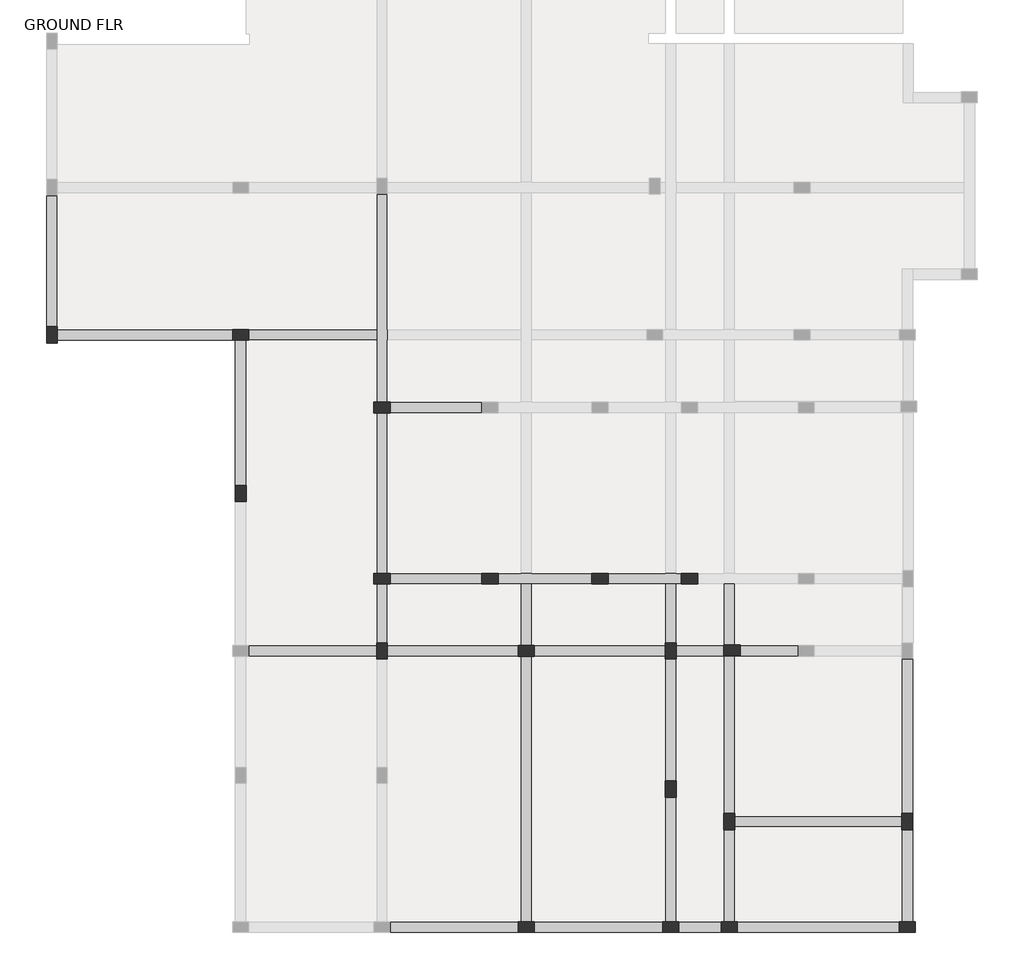
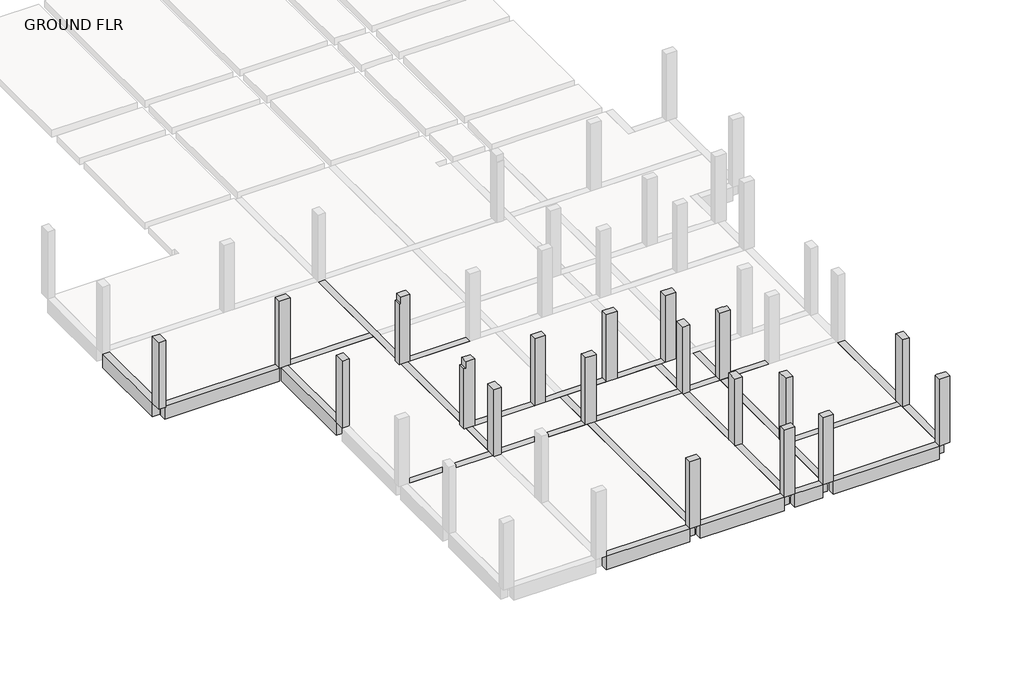
# One storey, part 2 of 5: 30 beams, 19 columns.
"""IFC4 building model written with IfcOpenShell, lengths in millimetres."""

from ifc_helpers import new_model, si_unit, frame, origin, place, context, project, spatial, polyline, outline, extrude, faceted_brep, element, save

model = new_model("IFC4")

# Units and contexts
model_context = context("Model", 3, world=origin())
ifc_project = project(units=[si_unit("LENGTHUNIT", "METRE", prefix="MILLI")], contexts=[model_context])

# Site, building, storey
site = spatial("IfcSite", under=ifc_project)
building = spatial("IfcBuilding", under=site)
storey = spatial("IfcBuildingStorey", under=building, Name="GROUND FLR", Elevation=0.0)

# Beams
placement = place(None, origin())
element("IfcBeam", 1, ObjectType="M_Concrete-Rectangular Beam : 300 x 600mm", at=placement, inside=storey, context=model_context, shape_type="SweptSolid", body=[
    extrude(outline(polyline([(-10828.8105653, -2764.4535766), (-11128.8105653, -2764.4535766), (-11128.8105653, 876.1713929), (-10828.8105653, 876.1713929), (-10828.8105653, -2764.4535766)])), frame((0.0, 0.0, -600.0), z_axis=(0.0, 0.0, 1.0), x_axis=(1.0, 0.0, 0.0)), (0.0, 0.0, 1.0), 600.0),
])
element("IfcBeam", 2, ObjectType="M_Concrete-Rectangular Beam : 300 x 600mm", at=placement, inside=storey, context=model_context, shape_type="Brep", body=[
    faceted_brep([(-5963.8105653, -3139.4535766, 0.0), (-5963.8105653, -2839.4535766, 0.0), (-10828.8105653, -2839.4535766, 0.0), (-10828.8105653, -3139.4535766, 0.0), (-5963.8105653, -3139.4535766, -600.0), (-10828.8105653, -3139.4535766, -600.0), (-5963.8105653, -2839.4535766, -600.0), (-10828.8105653, -2839.4535766, -600.0), (-5963.8105653, -2839.4535766, -300.0), (-10828.8105653, -2839.4535766, -300.0)], [[[0, 1, 2, 3]], [[4, 0, 3, 5]], [[6, 4, 5, 7]], [[2, 1, 8, 6, 7, 9]], [[1, 0, 4, 6, 8]], [[3, 2, 9, 7, 5]]]),
])
element("IfcBeam", 3, ObjectType="M_Concrete-Rectangular Beam : 300 x 600mm", at=placement, inside=storey, context=model_context, shape_type="Brep", body=[
    faceted_brep([(-5588.8105653, -7169.0760584, 0.0), (-5588.8105653, -3139.4535766, 0.0), (-5888.8105653, -3139.4535766, 0.0), (-5888.8105653, -7169.0760584, 0.0), (-5888.8105653, -3139.4535766, -600.0), (-5888.8105653, -7169.0760584, -600.0), (-5588.8105653, -3139.4535766, -600.0), (-5588.8105653, -7169.0760584, -600.0), (-5588.8105653, -7169.0760584, -300.0), (-5588.8105653, -3139.4535766, -300.0)], [[[0, 1, 2, 3]], [[3, 2, 4, 5]], [[5, 4, 6, 7]], [[1, 0, 8, 7, 6, 9]], [[6, 4, 2, 1, 9]], [[0, 3, 5, 7, 8]]]),
])
element("IfcBeam", 4, ObjectType="M_Concrete-Rectangular Beam : 300 x 600mm", at=placement, inside=storey, context=model_context, shape_type="SweptSolid", body=[
    extrude(outline(polyline([(1949.7296816, -19272.5304373), (1949.7296816, -19572.5304373), (-1596.7865686, -19572.5304373), (-1596.7865686, -19272.5304373), (1949.7296816, -19272.5304373)])), frame((0.0, 0.0, -600.0), z_axis=(0.0, 0.0, 1.0), x_axis=(1.0, 0.0, 0.0)), (0.0, 0.0, 1.0), 600.0),
])
element("IfcBeam", 5, ObjectType="M_Concrete-Rectangular Beam : 300 x 600mm", at=placement, inside=storey, context=model_context, shape_type="SweptSolid", body=[
    extrude(outline(polyline([(5957.5248054, -19272.5304373), (5957.5248054, -19572.5304373), (2399.7296816, -19572.5304373), (2399.7296816, -19272.5304373), (5957.5248054, -19272.5304373)])), frame((0.0, 0.0, -600.0), z_axis=(0.0, 0.0, 1.0), x_axis=(1.0, 0.0, 0.0)), (0.0, 0.0, 1.0), 600.0),
])
element("IfcBeam", 6, ObjectType="M_Concrete-Rectangular Beam : 300 x 600mm", at=placement, inside=storey, context=model_context, shape_type="SweptSolid", body=[
    extrude(outline(polyline([(7581.8679014, -19272.5304373), (7581.8679014, -19572.5304373), (6407.5248054, -19572.5304373), (6407.5248054, -19272.5304373), (7581.8679014, -19272.5304373)])), frame((0.0, 0.0, -600.0), z_axis=(0.0, 0.0, 1.0), x_axis=(1.0, 0.0, 0.0)), (0.0, 0.0, 1.0), 600.0),
])
element("IfcBeam", 7, ObjectType="M_Concrete-Rectangular Beam : 300 x 600mm", at=placement, inside=storey, context=model_context, shape_type="SweptSolid", body=[
    extrude(outline(polyline([(12524.1163908, -19272.5304373), (12524.1163908, -19572.5304373), (8031.8679014, -19572.5304373), (8031.8679014, -19272.5304373), (12524.1163908, -19272.5304373)])), frame((0.0, 0.0, -600.0), z_axis=(0.0, 0.0, 1.0), x_axis=(1.0, 0.0, 0.0)), (0.0, 0.0, 1.0), 600.0),
])
element("IfcBeam", 8, ObjectType="M_Concrete-Rectangular Beam : 300 x 600mm", at=placement, inside=storey, context=model_context, shape_type="Brep", body=[
    faceted_brep([(12599.1163908, -19272.5304373, 0.0), (12899.1163908, -19272.5304373, 0.0), (12899.1163908, -16719.1579597, 0.0), (12599.1163908, -16719.1579597, 0.0), (12899.1163908, -19272.5304373, -600.0), (12899.1163908, -16719.1579597, -600.0), (12599.1163908, -19272.5304373, -600.0), (12599.1163908, -16719.1579597, -600.0), (12599.1163908, -16719.1579597, -300.0), (12599.1163908, -19272.5304373, -300.0)], [[[0, 1, 2, 3]], [[1, 4, 5, 2]], [[4, 6, 7, 5]], [[0, 3, 8, 7, 6, 9]], [[6, 4, 1, 0, 9]], [[3, 2, 5, 7, 8]]]),
])
element("IfcBeam", 9, ObjectType="M_Concrete-Rectangular Beam : 300 x 600mm", at=placement, inside=storey, context=model_context, shape_type="Brep", body=[
    faceted_brep([(12599.1163908, -16269.1579597, 0.0), (12899.1163908, -16269.1579597, 0.0), (12899.1163908, -11982.8970059, 0.0), (12599.1163908, -11982.8970059, 0.0), (12899.1163908, -16269.1579597, -600.0), (12899.1163908, -11982.8970059, -600.0), (12599.1163908, -16269.1579597, -600.0), (12599.1163908, -11982.8970059, -600.0), (12599.1163908, -11982.8970059, -300.0), (12599.1163908, -16269.1579597, -300.0)], [[[0, 1, 2, 3]], [[1, 4, 5, 2]], [[4, 6, 7, 5]], [[0, 3, 8, 7, 6, 9]], [[6, 4, 1, 0, 9]], [[3, 2, 5, 7, 8]]]),
])
element("IfcBeam", 10, ObjectType="M_Concrete-Rectangular Beam : 300 x 600mm", at=placement, inside=storey, context=model_context, shape_type="Brep", body=[
    faceted_brep([(-1971.7865686, -9907.1078267, 0.0), (-1971.7865686, -11532.8970059, 0.0), (-1671.7865686, -11532.8970059, 0.0), (-1671.7865686, -9907.1078267, 0.0), (-1671.7865686, -11532.8970059, -300.0), (-1671.7865686, -11532.8970059, -600.0), (-1671.7865686, -9907.1078267, -600.0), (-1671.7865686, -9907.1078267, -300.0), (-1971.7865686, -11532.8970059, -600.0), (-1971.7865686, -9907.1078267, -600.0), (-1971.7865686, -9907.1078267, -300.0), (-1971.7865686, -11532.8970059, -300.0)], [[[0, 1, 2, 3]], [[3, 2, 4, 5, 6, 7]], [[6, 5, 8, 9]], [[1, 0, 10, 9, 8, 11]], [[0, 3, 7, 6, 9, 10]], [[8, 5, 4, 2, 1, 11]]]),
])
element("IfcBeam", 11, ObjectType="M_Concrete-Rectangular Beam : 300 x 600mm", at=placement, inside=storey, context=model_context, shape_type="Brep", body=[
    faceted_brep([(-1671.7865686, 916.1713929, 0.0), (-1971.7865686, 916.1713929, 0.0), (-1971.7865686, -2839.4535766, 0.0), (-1971.7865686, -3139.4535766, 0.0), (-1971.7865686, -4851.6229916, 0.0), (-1671.7865686, -4851.6229916, 0.0), (-1671.7865686, -3139.4535766, 0.0), (-1671.7865686, -2839.4535766, 0.0), (-1971.7865686, 916.1713929, -600.0), (-1971.7865686, -2839.4535766, -600.0), (-1971.7865686, -3139.4535766, -600.0), (-1971.7865686, -4851.6229916, -600.0), (-1971.7865686, -4851.6229916, -300.0), (-1971.7865686, 916.1713929, -300.0), (-1671.7865686, 916.1713929, -600.0), (-1671.7865686, -2839.4535766, -600.0), (-1671.7865686, -3139.4535766, -600.0), (-1671.7865686, -4851.6229916, -600.0), (-1671.7865686, 916.1713929, -300.0), (-1671.7865686, -4851.6229916, -300.0)], [[[0, 1, 2, 3, 4, 5, 6, 7]], [[8, 9, 10, 11, 12, 4, 3, 2, 1, 13]], [[8, 14, 15, 16, 17, 11, 10, 9]], [[17, 16, 15, 14, 18, 0, 7, 6, 5, 19]], [[1, 0, 18, 14, 8, 13]], [[5, 4, 12, 11, 17, 19]]]),
])
element("IfcBeam", 12, ObjectType="M_Concrete-Rectangular Beam : 300 x 600mm", at=placement, inside=storey, context=model_context, shape_type="Brep", body=[
    faceted_brep([(-1671.7865686, -5151.6229916, 0.0), (-1971.7865686, -5151.6229916, 0.0), (-1971.7865686, -9607.1078267, 0.0), (-1671.7865686, -9607.1078267, 0.0), (-1971.7865686, -5151.6229916, -300.0), (-1971.7865686, -5151.6229916, -600.0), (-1971.7865686, -9607.1078267, -600.0), (-1971.7865686, -9607.1078267, -300.0), (-1671.7865686, -5151.6229916, -600.0), (-1671.7865686, -9607.1078267, -600.0), (-1671.7865686, -9607.1078267, -300.0), (-1671.7865686, -5151.6229916, -300.0)], [[[0, 1, 2, 3]], [[2, 1, 4, 5, 6, 7]], [[5, 8, 9, 6]], [[0, 3, 10, 9, 8, 11]], [[1, 0, 11, 8, 5, 4]], [[3, 2, 7, 6, 9, 10]]]),
])
element("IfcBeam", 13, ObjectType="M_Concrete-Rectangular Beam : 300 x 600mm", at=placement, inside=storey, context=model_context, shape_type="Brep", body=[
    faceted_brep([(2324.7296816, -11907.8970059, 0.0), (2024.7296816, -11907.8970059, 0.0), (2024.7296816, -19272.5304373, 0.0), (2324.7296816, -19272.5304373, 0.0), (2024.7296816, -11907.8970059, -300.0), (2024.7296816, -11907.8970059, -600.0), (2024.7296816, -19272.5304373, -600.0), (2024.7296816, -19272.5304373, -300.0), (2324.7296816, -11907.8970059, -600.0), (2324.7296816, -19272.5304373, -600.0), (2324.7296816, -19272.5304373, -300.0), (2324.7296816, -11907.8970059, -300.0)], [[[0, 1, 2, 3]], [[2, 1, 4, 5, 6, 7]], [[5, 8, 9, 6]], [[0, 3, 10, 9, 8, 11]], [[1, 0, 11, 8, 5, 4]], [[3, 2, 7, 6, 9, 10]]]),
])
element("IfcBeam", 14, ObjectType="M_Concrete-Rectangular Beam : 300 x 600mm", at=placement, inside=storey, context=model_context, shape_type="Brep", body=[
    faceted_brep([(6332.5248054, -11982.8970059, 0.0), (6032.5248054, -11982.8970059, 0.0), (6032.5248054, -15369.1579597, 0.0), (6332.5248054, -15369.1579597, 0.0), (6032.5248054, -11982.8970059, -300.0), (6032.5248054, -11982.8970059, -600.0), (6032.5248054, -15369.1579597, -600.0), (6032.5248054, -15369.1579597, -300.0), (6332.5248054, -11982.8970059, -600.0), (6332.5248054, -15369.1579597, -600.0), (6332.5248054, -15369.1579597, -300.0), (6332.5248054, -11982.8970059, -300.0)], [[[0, 1, 2, 3]], [[2, 1, 4, 5, 6, 7]], [[5, 8, 9, 6]], [[0, 3, 10, 9, 8, 11]], [[1, 0, 11, 8, 5, 4]], [[3, 2, 7, 6, 9, 10]]]),
])
element("IfcBeam", 15, ObjectType="M_Concrete-Rectangular Beam : 300 x 600mm", at=placement, inside=storey, context=model_context, shape_type="Brep", body=[
    faceted_brep([(6032.5248054, -19272.5304373, 0.0), (6332.5248054, -19272.5304373, 0.0), (6332.5248054, -15819.1579597, 0.0), (6032.5248054, -15819.1579597, 0.0), (6032.5248054, -15819.1579597, -300.0), (6032.5248054, -15819.1579597, -600.0), (6032.5248054, -19272.5304373, -600.0), (6032.5248054, -19272.5304373, -300.0), (6332.5248054, -19272.5304373, -600.0), (6332.5248054, -15819.1579597, -600.0), (6332.5248054, -19272.5304373, -300.0), (6332.5248054, -15819.1579597, -300.0)], [[[0, 1, 2, 3]], [[0, 3, 4, 5, 6, 7]], [[8, 6, 5, 9]], [[2, 1, 10, 8, 9, 11]], [[1, 0, 7, 6, 8, 10]], [[3, 2, 11, 9, 5, 4]]]),
])
element("IfcBeam", 16, ObjectType="M_Concrete-Rectangular Beam : 300 x 600mm", at=placement, inside=storey, context=model_context, shape_type="Brep", body=[
    faceted_brep([(7656.8679014, -19272.5304373, 0.0), (7956.8679014, -19272.5304373, 0.0), (7956.8679014, -16719.1579597, 0.0), (7656.8679014, -16719.1579597, 0.0), (7656.8679014, -16719.1579597, -300.0), (7656.8679014, -16719.1579597, -600.0), (7656.8679014, -19272.5304373, -600.0), (7656.8679014, -19272.5304373, -300.0), (7956.8679014, -19272.5304373, -600.0), (7956.8679014, -16719.1579597, -600.0), (7956.8679014, -19272.5304373, -300.0), (7956.8679014, -16719.1579597, -300.0)], [[[0, 1, 2, 3]], [[0, 3, 4, 5, 6, 7]], [[8, 6, 5, 9]], [[2, 1, 10, 8, 9, 11]], [[1, 0, 7, 6, 8, 10]], [[3, 2, 11, 9, 5, 4]]]),
])
element("IfcBeam", 17, ObjectType="M_Concrete-Rectangular Beam : 300 x 600mm", at=placement, inside=storey, context=model_context, shape_type="Brep", body=[
    faceted_brep([(-5513.8105653, -2839.4535766, 0.0), (-5513.8105653, -3139.4535766, 0.0), (-1971.7865686, -3139.4535766, 0.0), (-1971.7865686, -2839.4535766, 0.0), (-5513.8105653, -3139.4535766, -300.0), (-5513.8105653, -3139.4535766, -600.0), (-1971.7865686, -3139.4535766, -600.0), (-1971.7865686, -3139.4535766, -300.0), (-5513.8105653, -2839.4535766, -600.0), (-1971.7865686, -2839.4535766, -600.0), (-1971.7865686, -2839.4535766, -300.0), (-5513.8105653, -2839.4535766, -300.0)], [[[0, 1, 2, 3]], [[2, 1, 4, 5, 6, 7]], [[5, 8, 9, 6]], [[0, 3, 10, 9, 8, 11]], [[1, 0, 11, 8, 5, 4]], [[3, 2, 7, 6, 9, 10]]]),
])
element("IfcBeam", 18, ObjectType="M_Concrete-Rectangular Beam : 300 x 600mm", at=placement, inside=storey, context=model_context, shape_type="Brep", body=[
    faceted_brep([(-1596.7865686, -4851.6229916, 0.0), (-1596.7865686, -5151.6229916, 0.0), (949.7296816, -5151.6229916, 0.0), (949.7296816, -4851.6229916, 0.0), (-1596.7865686, -5151.6229916, -300.0), (-1596.7865686, -5151.6229916, -600.0), (949.7296816, -5151.6229916, -600.0), (949.7296816, -5151.6229916, -300.0), (-1596.7865686, -4851.6229916, -600.0), (949.7296816, -4851.6229916, -600.0), (949.7296816, -4851.6229916, -300.0), (-1596.7865686, -4851.6229916, -300.0)], [[[0, 1, 2, 3]], [[2, 1, 4, 5, 6, 7]], [[5, 8, 9, 6]], [[0, 3, 10, 9, 8, 11]], [[1, 0, 11, 8, 5, 4]], [[3, 2, 7, 6, 9, 10]]]),
])
element("IfcBeam", 19, ObjectType="M_Concrete-Rectangular Beam : 300 x 600mm", at=placement, inside=storey, context=model_context, shape_type="Brep", body=[
    faceted_brep([(-1971.7865686, -11907.8970059, 0.0), (-1971.7865686, -11607.8970059, 0.0), (-5513.8105653, -11607.8970059, 0.0), (-5513.8105653, -11907.8970059, 0.0), (-5513.8105653, -11907.8970059, -300.0), (-5513.8105653, -11907.8970059, -600.0), (-1971.7865686, -11907.8970059, -600.0), (-1971.7865686, -11907.8970059, -300.0), (-1971.7865686, -11607.8970059, -600.0), (-5513.8105653, -11607.8970059, -600.0), (-1971.7865686, -11607.8970059, -300.0), (-5513.8105653, -11607.8970059, -300.0)], [[[0, 1, 2, 3]], [[0, 3, 4, 5, 6, 7]], [[8, 6, 5, 9]], [[2, 1, 10, 8, 9, 11]], [[1, 0, 7, 6, 8, 10]], [[3, 2, 11, 9, 5, 4]]]),
])
element("IfcBeam", 20, ObjectType="M_Concrete-Rectangular Beam : 300 x 600mm", at=placement, inside=storey, context=model_context, shape_type="Brep", body=[
    faceted_brep([(1949.7296816, -11907.8970059, 0.0), (1949.7296816, -11607.8970059, 0.0), (-1671.7865686, -11607.8970059, 0.0), (-1671.7865686, -11907.8970059, 0.0), (-1671.7865686, -11907.8970059, -300.0), (-1671.7865686, -11907.8970059, -600.0), (1949.7296816, -11907.8970059, -600.0), (1949.7296816, -11907.8970059, -300.0), (1949.7296816, -11607.8970059, -600.0), (-1671.7865686, -11607.8970059, -600.0), (1949.7296816, -11607.8970059, -300.0), (-1671.7865686, -11607.8970059, -300.0)], [[[0, 1, 2, 3]], [[0, 3, 4, 5, 6, 7]], [[8, 6, 5, 9]], [[2, 1, 10, 8, 9, 11]], [[1, 0, 7, 6, 8, 10]], [[3, 2, 11, 9, 5, 4]]]),
])
element("IfcBeam", 21, ObjectType="M_Concrete-Rectangular Beam : 300 x 600mm", at=placement, inside=storey, context=model_context, shape_type="Brep", body=[
    faceted_brep([(6032.5248054, -11907.8970059, 0.0), (6032.5248054, -11607.8970059, 0.0), (2399.7296816, -11607.8970059, 0.0), (2399.7296816, -11907.8970059, 0.0), (2399.7296816, -11907.8970059, -300.0), (2399.7296816, -11907.8970059, -600.0), (6032.5248054, -11907.8970059, -600.0), (6032.5248054, -11907.8970059, -300.0), (6032.5248054, -11607.8970059, -600.0), (2399.7296816, -11607.8970059, -600.0), (6032.5248054, -11607.8970059, -300.0), (2399.7296816, -11607.8970059, -300.0)], [[[0, 1, 2, 3]], [[0, 3, 4, 5, 6, 7]], [[8, 6, 5, 9]], [[2, 1, 10, 8, 9, 11]], [[1, 0, 7, 6, 8, 10]], [[3, 2, 11, 9, 5, 4]]]),
])
element("IfcBeam", 22, ObjectType="M_Concrete-Rectangular Beam : 300 x 600mm", at=placement, inside=storey, context=model_context, shape_type="Brep", body=[
    faceted_brep([(9721.8679014, -11907.8970059, 0.0), (9721.8679014, -11607.8970059, 0.0), (8111.8679014, -11607.8970059, 0.0), (8111.8679014, -11887.8970059, 0.0), (7661.8679014, -11887.8970059, 0.0), (7661.8679014, -11607.8970059, 0.0), (7656.8679014, -11607.8970059, 0.0), (6332.5248054, -11607.8970059, 0.0), (6332.5248054, -11907.8970059, 0.0), (7656.8679014, -11907.8970059, 0.0), (7956.8679014, -11907.8970059, 0.0), (6332.5248054, -11907.8970059, -600.0), (7656.8679014, -11907.8970059, -600.0), (7956.8679014, -11907.8970059, -600.0), (9721.8679014, -11907.8970059, -600.0), (9721.8679014, -11907.8970059, -300.0), (6332.5248054, -11907.8970059, -300.0), (9721.8679014, -11607.8970059, -600.0), (6332.5248054, -11607.8970059, -600.0), (7656.8679014, -11607.8970059, -600.0), (7661.8679014, -11607.8970059, -600.0), (7661.8679014, -11887.8970059, -600.0), (8111.8679014, -11887.8970059, -600.0), (8111.8679014, -11607.8970059, -600.0), (6332.5248054, -11607.8970059, -300.0), (9721.8679014, -11607.8970059, -300.0), (8111.8679014, -11607.8970059, -300.0)], [[[0, 1, 2, 3, 4, 5, 6, 7, 8, 9, 10]], [[11, 12, 13, 14, 15, 0, 10, 9, 8, 16]], [[17, 14, 13, 12, 11, 18, 19, 20, 21, 22, 23]], [[20, 19, 18, 24, 7, 6, 5]], [[1, 0, 15, 14, 17, 25]], [[8, 7, 24, 18, 11, 16]], [[22, 3, 2, 26, 23]], [[3, 22, 21, 4]], [[4, 21, 20, 5]], [[2, 1, 25, 17, 23, 26]]]),
])
element("IfcBeam", 23, ObjectType="M_Concrete-Rectangular Beam : 300 x 600mm", at=placement, inside=storey, context=model_context, shape_type="Brep", body=[
    faceted_brep([(12599.1163908, -16644.1579597, 0.0), (12599.1163908, -16344.1579597, 0.0), (7956.8679014, -16344.1579597, 0.0), (7956.8679014, -16644.1579597, 0.0), (7956.8679014, -16644.1579597, -300.0), (7956.8679014, -16644.1579597, -600.0), (12599.1163908, -16644.1579597, -600.0), (12599.1163908, -16644.1579597, -300.0), (12599.1163908, -16344.1579597, -600.0), (7956.8679014, -16344.1579597, -600.0), (12599.1163908, -16344.1579597, -300.0), (7956.8679014, -16344.1579597, -300.0)], [[[0, 1, 2, 3]], [[0, 3, 4, 5, 6, 7]], [[8, 6, 5, 9]], [[2, 1, 10, 8, 9, 11]], [[1, 0, 7, 6, 8, 10]], [[3, 2, 11, 9, 5, 4]]]),
])
element("IfcBeam", 24, ObjectType="M_Concrete-Rectangular Beam : 300 x 600mm", at=placement, inside=storey, context=model_context, shape_type="Brep", body=[
    faceted_brep([(-1596.7865686, -9607.1078267, 0.0), (-1596.7865686, -9907.1078267, 0.0), (949.7296816, -9907.1078267, 0.0), (949.7296816, -9607.1078267, 0.0), (-1596.7865686, -9907.1078267, -300.0), (-1596.7865686, -9907.1078267, -600.0), (949.7296816, -9907.1078267, -600.0), (949.7296816, -9907.1078267, -300.0), (-1596.7865686, -9607.1078267, -600.0), (949.7296816, -9607.1078267, -600.0), (949.7296816, -9607.1078267, -300.0), (-1596.7865686, -9607.1078267, -300.0)], [[[0, 1, 2, 3]], [[2, 1, 4, 5, 6, 7]], [[5, 8, 9, 6]], [[0, 3, 10, 9, 8, 11]], [[1, 0, 11, 8, 5, 4]], [[3, 2, 7, 6, 9, 10]]]),
])
element("IfcBeam", 25, ObjectType="M_Concrete-Rectangular Beam : 300 x 600mm", at=placement, inside=storey, context=model_context, shape_type="Brep", body=[
    faceted_brep([(1399.7296816, -9607.1078267, 0.0), (1399.7296816, -9907.1078267, 0.0), (2024.7296816, -9907.1078267, 0.0), (2324.7296816, -9907.1078267, 0.0), (3997.5248054, -9907.1078267, 0.0), (3997.5248054, -9607.1078267, 0.0), (2324.7296816, -9607.1078267, 0.0), (2024.7296816, -9607.1078267, 0.0), (1399.7296816, -9907.1078267, -600.0), (2024.7296816, -9907.1078267, -600.0), (2324.7296816, -9907.1078267, -600.0), (3997.5248054, -9907.1078267, -600.0), (3997.5248054, -9907.1078267, -300.0), (1399.7296816, -9907.1078267, -300.0), (1399.7296816, -9607.1078267, -600.0), (2024.7296816, -9607.1078267, -600.0), (2324.7296816, -9607.1078267, -600.0), (3997.5248054, -9607.1078267, -600.0), (1399.7296816, -9607.1078267, -300.0), (3997.5248054, -9607.1078267, -300.0)], [[[0, 1, 2, 3, 4, 5, 6, 7]], [[8, 9, 10, 11, 12, 4, 3, 2, 1, 13]], [[8, 14, 15, 16, 17, 11, 10, 9]], [[17, 16, 15, 14, 18, 0, 7, 6, 5, 19]], [[1, 0, 18, 14, 8, 13]], [[5, 4, 12, 11, 17, 19]]]),
])
element("IfcBeam", 26, ObjectType="M_Concrete-Rectangular Beam : 300 x 600mm", at=placement, inside=storey, context=model_context, shape_type="Brep", body=[
    faceted_brep([(4447.5248054, -9607.1078267, 0.0), (4447.5248054, -9907.1078267, 0.0), (6032.5248054, -9907.1078267, 0.0), (6332.5248054, -9907.1078267, 0.0), (6481.8679014, -9907.1078267, 0.0), (6481.8679014, -9607.1078267, 0.0), (6332.5248054, -9607.1078267, 0.0), (6032.5248054, -9607.1078267, 0.0), (4447.5248054, -9907.1078267, -600.0), (6032.5248054, -9907.1078267, -600.0), (6332.5248054, -9907.1078267, -600.0), (6481.8679014, -9907.1078267, -600.0), (6481.8679014, -9907.1078267, -300.0), (4447.5248054, -9907.1078267, -300.0), (4447.5248054, -9607.1078267, -600.0), (6032.5248054, -9607.1078267, -600.0), (6332.5248054, -9607.1078267, -600.0), (6481.8679014, -9607.1078267, -600.0), (4447.5248054, -9607.1078267, -300.0), (6481.8679014, -9607.1078267, -300.0)], [[[0, 1, 2, 3, 4, 5, 6, 7]], [[8, 9, 10, 11, 12, 4, 3, 2, 1, 13]], [[8, 14, 15, 16, 17, 11, 10, 9]], [[17, 16, 15, 14, 18, 0, 7, 6, 5, 19]], [[1, 0, 18, 14, 8, 13]], [[5, 4, 12, 11, 17, 19]]]),
])
element("IfcBeam", 27, ObjectType="M_Concrete-Rectangular Beam : 300 x 600mm", at=placement, inside=storey, context=model_context, shape_type="Brep", body=[
    faceted_brep([(7656.8679014, -16269.1579597, 0.0), (7956.8679014, -16269.1579597, 0.0), (7956.8679014, -11907.8970059, 0.0), (7656.8679014, -11907.8970059, 0.0), (7656.8679014, -11907.8970059, -300.0), (7656.8679014, -11907.8970059, -600.0), (7656.8679014, -16269.1579597, -600.0), (7656.8679014, -16269.1579597, -300.0), (7956.8679014, -16269.1579597, -600.0), (7956.8679014, -11907.8970059, -600.0), (7956.8679014, -16269.1579597, -300.0), (7956.8679014, -11907.8970059, -300.0)], [[[0, 1, 2, 3]], [[0, 3, 4, 5, 6, 7]], [[8, 6, 5, 9]], [[2, 1, 10, 8, 9, 11]], [[1, 0, 7, 6, 8, 10]], [[3, 2, 11, 9, 5, 4]]]),
])
element("IfcBeam", 28, ObjectType="M_Concrete-Rectangular Beam : 300 x 600mm", at=placement, inside=storey, context=model_context, shape_type="Brep", body=[
    faceted_brep([(2024.7296816, -11607.8970059, 0.0), (2324.7296816, -11607.8970059, 0.0), (2324.7296816, -9907.1078267, 0.0), (2024.7296816, -9907.1078267, 0.0), (2024.7296816, -9907.1078267, -300.0), (2024.7296816, -9907.1078267, -600.0), (2024.7296816, -11607.8970059, -600.0), (2024.7296816, -11607.8970059, -300.0), (2324.7296816, -11607.8970059, -600.0), (2324.7296816, -9907.1078267, -600.0), (2324.7296816, -11607.8970059, -300.0), (2324.7296816, -9907.1078267, -300.0)], [[[0, 1, 2, 3]], [[0, 3, 4, 5, 6, 7]], [[8, 6, 5, 9]], [[2, 1, 10, 8, 9, 11]], [[1, 0, 7, 6, 8, 10]], [[3, 2, 11, 9, 5, 4]]]),
])
element("IfcBeam", 29, ObjectType="M_Concrete-Rectangular Beam : 300 x 600mm", at=placement, inside=storey, context=model_context, shape_type="Brep", body=[
    faceted_brep([(6032.5248054, -11532.8970059, 0.0), (6332.5248054, -11532.8970059, 0.0), (6332.5248054, -9907.1078267, 0.0), (6032.5248054, -9907.1078267, 0.0), (6032.5248054, -9907.1078267, -300.0), (6032.5248054, -9907.1078267, -600.0), (6032.5248054, -11532.8970059, -600.0), (6032.5248054, -11532.8970059, -300.0), (6332.5248054, -11532.8970059, -600.0), (6332.5248054, -9907.1078267, -600.0), (6332.5248054, -11532.8970059, -300.0), (6332.5248054, -9907.1078267, -300.0)], [[[0, 1, 2, 3]], [[0, 3, 4, 5, 6, 7]], [[8, 6, 5, 9]], [[2, 1, 10, 8, 9, 11]], [[1, 0, 7, 6, 8, 10]], [[3, 2, 11, 9, 5, 4]]]),
])
element("IfcBeam", 30, ObjectType="M_Concrete-Rectangular Beam : 300 x 600mm", at=placement, inside=storey, context=model_context, shape_type="Brep", body=[
    faceted_brep([(7661.8679014, -11587.8970059, 0.0), (7956.8679014, -11587.8970059, 0.0), (7956.8679014, -9907.1078267, 0.0), (7656.8679014, -9907.1078267, 0.0), (7656.8679014, -11607.8970059, 0.0), (7661.8679014, -11607.8970059, 0.0), (7656.8679014, -9907.1078267, -300.0), (7656.8679014, -9907.1078267, -600.0), (7656.8679014, -11607.8970059, -600.0), (7656.8679014, -11607.8970059, -300.0), (7956.8679014, -11587.8970059, -600.0), (7661.8679014, -11587.8970059, -600.0), (7661.8679014, -11607.8970059, -600.0), (7956.8679014, -9907.1078267, -600.0), (7956.8679014, -11587.8970059, -300.0), (7956.8679014, -9907.1078267, -300.0)], [[[0, 1, 2, 3, 4, 5]], [[4, 3, 6, 7, 8, 9]], [[10, 11, 12, 8, 7, 13]], [[2, 1, 14, 10, 13, 15]], [[0, 11, 10, 14, 1]], [[11, 0, 5, 12]], [[3, 2, 15, 13, 7, 6]], [[5, 4, 9, 8, 12]]]),
])

# Columns
element("IfcColumn", 31, ObjectType="M_Concrete-Rectangular-Column : 300 x 450mm", at=placement, inside=storey, context=model_context, shape_type="Brep", body=[
    faceted_brep([(-11128.8105653, -3214.4535766, 0.0), (-11128.8105653, -2764.4535766, 0.0), (-10828.8105653, -2764.4535766, 0.0), (-10828.8105653, -3214.4535766, 0.0), (-11128.8105653, -3214.4535766, 3000.0), (-11128.8105653, -2764.4535766, 3000.0), (-10828.8105653, -2764.4535766, 3000.0), (-10828.8105653, -2839.4535766, 3000.0), (-10828.8105653, -3214.4535766, 3000.0)], [[[0, 1, 2, 3]], [[4, 5, 1, 0]], [[5, 6, 2, 1]], [[6, 7, 8, 3, 2]], [[8, 4, 0, 3]], [[4, 8, 7, 6, 5]]]),
])
element("IfcColumn", 32, ObjectType="M_Concrete-Rectangular-Column : 300 x 450mm", at=placement, inside=storey, context=model_context, shape_type="Brep", body=[
    faceted_brep([(-5513.8105653, -3139.4535766, 0.0), (-5963.8105653, -3139.4535766, 0.0), (-5963.8105653, -2839.4535766, 0.0), (-5513.8105653, -2839.4535766, 0.0), (-5513.8105653, -3139.4535766, 2700.0), (-5513.8105653, -3139.4535766, 3000.0), (-5588.8105653, -3139.4535766, 3000.0), (-5963.8105653, -3139.4535766, 3000.0), (-5963.8105653, -2839.4535766, 3000.0), (-5963.8105653, -2839.4535766, 2700.0), (-5513.8105653, -2839.4535766, 3000.0), (-5513.8105653, -2839.4535766, 2700.0)], [[[0, 1, 2, 3]], [[1, 0, 4, 5, 6, 7]], [[2, 1, 7, 8, 9]], [[3, 2, 9, 8, 10, 11]], [[0, 3, 11, 10, 5, 4]], [[8, 7, 6, 5, 10]]]),
])
element("IfcColumn", 33, ObjectType="M_Concrete-Rectangular-Column : 300 x 450mm", at=placement, inside=storey, context=model_context, shape_type="Brep", body=[
    faceted_brep([(-1596.7865686, -5151.6229916, 0.0), (-2046.7865686, -5151.6229916, 0.0), (-2046.7865686, -4851.6229916, 0.0), (-1596.7865686, -4851.6229916, 0.0), (-1596.7865686, -5151.6229916, 2700.0), (-1596.7865686, -5151.6229916, 3000.0), (-1671.7865686, -5151.6229916, 3000.0), (-1971.7865686, -5151.6229916, 3000.0), (-1971.7865686, -5151.6229916, 2700.0), (-2046.7865686, -5151.6229916, 2700.0), (-2046.7865686, -4851.6229916, 2700.0), (-1971.7865686, -4851.6229916, 2700.0), (-1971.7865686, -4851.6229916, 3000.0), (-1671.7865686, -4851.6229916, 3000.0), (-1596.7865686, -4851.6229916, 3000.0), (-1596.7865686, -4851.6229916, 2700.0)], [[[0, 1, 2, 3]], [[1, 0, 4, 5, 6, 7, 8, 9]], [[2, 1, 9, 10]], [[3, 2, 10, 11, 12, 13, 14, 15]], [[0, 3, 15, 14, 5, 4]], [[5, 14, 13, 12, 7, 6]], [[8, 11, 10, 9]], [[11, 8, 7, 12]]]),
])
element("IfcColumn", 34, ObjectType="M_Concrete-Rectangular-Column : 300 x 450mm", at=placement, inside=storey, context=model_context, shape_type="Brep", body=[
    faceted_brep([(-1596.7865686, -9907.1078267, 0.0), (-2046.7865686, -9907.1078267, 0.0), (-2046.7865686, -9607.1078267, 0.0), (-1596.7865686, -9607.1078267, 0.0), (-1596.7865686, -9907.1078267, 2700.0), (-1596.7865686, -9907.1078267, 3000.0), (-1671.7865686, -9907.1078267, 3000.0), (-1971.7865686, -9907.1078267, 3000.0), (-1971.7865686, -9907.1078267, 2700.0), (-2046.7865686, -9907.1078267, 2700.0), (-2046.7865686, -9607.1078267, 2700.0), (-1971.7865686, -9607.1078267, 2700.0), (-1971.7865686, -9607.1078267, 3000.0), (-1671.7865686, -9607.1078267, 3000.0), (-1596.7865686, -9607.1078267, 3000.0), (-1596.7865686, -9607.1078267, 2700.0)], [[[0, 1, 2, 3]], [[1, 0, 4, 5, 6, 7, 8, 9]], [[2, 1, 9, 10]], [[3, 2, 10, 11, 12, 13, 14, 15]], [[0, 3, 15, 14, 5, 4]], [[5, 14, 13, 12, 7, 6]], [[8, 11, 10, 9]], [[11, 8, 7, 12]]]),
])
element("IfcColumn", 35, ObjectType="M_Concrete-Rectangular-Column : 300 x 450mm", at=placement, inside=storey, context=model_context, shape_type="Brep", body=[
    faceted_brep([(1399.7296816, -9907.1078267, 0.0), (949.7296816, -9907.1078267, 0.0), (949.7296816, -9607.1078267, 0.0), (1399.7296816, -9607.1078267, 0.0), (1399.7296816, -9907.1078267, 2700.0), (1399.7296816, -9907.1078267, 3000.0), (949.7296816, -9907.1078267, 3000.0), (949.7296816, -9907.1078267, 2700.0), (949.7296816, -9607.1078267, 3000.0), (949.7296816, -9607.1078267, 2700.0), (1399.7296816, -9607.1078267, 3000.0), (1399.7296816, -9607.1078267, 2700.0)], [[[0, 1, 2, 3]], [[1, 0, 4, 5, 6, 7]], [[2, 1, 7, 6, 8, 9]], [[3, 2, 9, 8, 10, 11]], [[0, 3, 11, 10, 5, 4]], [[6, 5, 10, 8]]]),
])
element("IfcColumn", 36, ObjectType="M_Concrete-Rectangular-Column : 300 x 450mm", at=placement, inside=storey, context=model_context, shape_type="Brep", body=[
    faceted_brep([(4447.5248054, -9907.1078267, 0.0), (3997.5248054, -9907.1078267, 0.0), (3997.5248054, -9607.1078267, 0.0), (4447.5248054, -9607.1078267, 0.0), (4447.5248054, -9907.1078267, 2700.0), (4447.5248054, -9907.1078267, 3000.0), (3997.5248054, -9907.1078267, 3000.0), (3997.5248054, -9907.1078267, 2700.0), (3997.5248054, -9607.1078267, 3000.0), (3997.5248054, -9607.1078267, 2700.0), (4447.5248054, -9607.1078267, 3000.0), (4447.5248054, -9607.1078267, 2700.0)], [[[0, 1, 2, 3]], [[1, 0, 4, 5, 6, 7]], [[2, 1, 7, 6, 8, 9]], [[3, 2, 9, 8, 10, 11]], [[0, 3, 11, 10, 5, 4]], [[6, 5, 10, 8]]]),
])
element("IfcColumn", 37, ObjectType="M_Concrete-Rectangular-Column : 300 x 450mm", at=placement, inside=storey, context=model_context, shape_type="Brep", body=[
    faceted_brep([(6931.8679014, -9907.1078267, 0.0), (6481.8679014, -9907.1078267, 0.0), (6481.8679014, -9607.1078267, 0.0), (6931.8679014, -9607.1078267, 0.0), (6931.8679014, -9907.1078267, 2700.0), (6931.8679014, -9907.1078267, 3000.0), (6481.8679014, -9907.1078267, 3000.0), (6481.8679014, -9907.1078267, 2700.0), (6481.8679014, -9607.1078267, 3000.0), (6481.8679014, -9607.1078267, 2700.0), (6931.8679014, -9607.1078267, 3000.0), (6931.8679014, -9607.1078267, 2700.0)], [[[0, 1, 2, 3]], [[1, 0, 4, 5, 6, 7]], [[2, 1, 7, 6, 8, 9]], [[3, 2, 9, 8, 10, 11]], [[0, 3, 11, 10, 5, 4]], [[6, 5, 10, 8]]]),
])
element("IfcColumn", 38, ObjectType="M_Concrete-Rectangular-Column : 300 x 450mm", at=placement, inside=storey, context=model_context, shape_type="Brep", body=[
    faceted_brep([(7661.8679014, -11587.8970059, 0.0), (8111.8679014, -11587.8970059, 0.0), (8111.8679014, -11887.8970059, 0.0), (7661.8679014, -11887.8970059, 0.0), (7661.8679014, -11587.8970059, 3000.0), (7956.8679014, -11587.8970059, 3000.0), (7956.8679014, -11587.8970059, 2700.0), (8111.8679014, -11587.8970059, 2700.0), (8111.8679014, -11607.8970059, 2700.0), (8111.8679014, -11607.8970059, 3000.0), (8111.8679014, -11887.8970059, 3000.0), (8111.8679014, -11887.8970059, 2400.0), (7661.8679014, -11887.8970059, 3000.0), (7661.8679014, -11887.8970059, 2400.0), (7661.8679014, -11607.8970059, 3000.0), (7956.8679014, -11607.8970059, 3000.0), (7956.8679014, -11607.8970059, 2700.0)], [[[0, 1, 2, 3]], [[1, 0, 4, 5, 6, 7]], [[2, 1, 7, 8, 9, 10, 11]], [[3, 2, 11, 10, 12, 13]], [[0, 3, 13, 12, 14, 4]], [[12, 10, 9, 15, 5, 4, 14]], [[6, 16, 8, 7]], [[16, 15, 9, 8]], [[15, 16, 6, 5]]]),
])
element("IfcColumn", 39, ObjectType="M_Concrete-Rectangular-Column : 300 x 450mm", at=placement, inside=storey, context=model_context, shape_type="Brep", body=[
    faceted_brep([(6332.5248054, -11532.8970059, 0.0), (6332.5248054, -11982.8970059, 0.0), (6032.5248054, -11982.8970059, 0.0), (6032.5248054, -11532.8970059, 0.0), (6332.5248054, -11532.8970059, 2700.0), (6332.5248054, -11532.8970059, 3000.0), (6332.5248054, -11607.8970059, 3000.0), (6332.5248054, -11907.8970059, 3000.0), (6332.5248054, -11982.8970059, 3000.0), (6332.5248054, -11982.8970059, 2700.0), (6032.5248054, -11982.8970059, 3000.0), (6032.5248054, -11982.8970059, 2700.0), (6032.5248054, -11907.8970059, 3000.0), (6032.5248054, -11607.8970059, 3000.0), (6032.5248054, -11532.8970059, 3000.0), (6032.5248054, -11532.8970059, 2700.0)], [[[0, 1, 2, 3]], [[1, 0, 4, 5, 6, 7, 8, 9]], [[2, 1, 9, 8, 10, 11]], [[3, 2, 11, 10, 12, 13, 14, 15]], [[0, 3, 15, 14, 5, 4]], [[10, 8, 7, 6, 5, 14, 13, 12]]]),
])
element("IfcColumn", 40, ObjectType="M_Concrete-Rectangular-Column : 300 x 450mm", at=placement, inside=storey, context=model_context, shape_type="Brep", body=[
    faceted_brep([(1949.7296816, -11607.8970059, 0.0), (2399.7296816, -11607.8970059, 0.0), (2399.7296816, -11907.8970059, 0.0), (1949.7296816, -11907.8970059, 0.0), (1949.7296816, -11607.8970059, 2700.0), (1949.7296816, -11607.8970059, 3000.0), (2024.7296816, -11607.8970059, 3000.0), (2324.7296816, -11607.8970059, 3000.0), (2399.7296816, -11607.8970059, 3000.0), (2399.7296816, -11607.8970059, 2700.0), (2399.7296816, -11907.8970059, 3000.0), (2399.7296816, -11907.8970059, 2700.0), (2324.7296816, -11907.8970059, 3000.0), (2024.7296816, -11907.8970059, 3000.0), (1949.7296816, -11907.8970059, 3000.0), (1949.7296816, -11907.8970059, 2700.0)], [[[0, 1, 2, 3]], [[1, 0, 4, 5, 6, 7, 8, 9]], [[2, 1, 9, 8, 10, 11]], [[3, 2, 11, 10, 12, 13, 14, 15]], [[0, 3, 15, 14, 5, 4]], [[10, 8, 7, 6, 5, 14, 13, 12]]]),
])
element("IfcColumn", 41, ObjectType="M_Concrete-Rectangular-Column : 300 x 450mm", at=placement, inside=storey, context=model_context, shape_type="Brep", body=[
    faceted_brep([(-1971.7865686, -11982.8970059, 0.0), (-1971.7865686, -11532.8970059, 0.0), (-1671.7865686, -11532.8970059, 0.0), (-1671.7865686, -11982.8970059, 0.0), (-1971.7865686, -11982.8970059, 2700.0), (-1971.7865686, -11982.8970059, 3000.0), (-1971.7865686, -11907.8970059, 3000.0), (-1971.7865686, -11607.8970059, 3000.0), (-1971.7865686, -11532.8970059, 3000.0), (-1971.7865686, -11532.8970059, 2700.0), (-1671.7865686, -11532.8970059, 3000.0), (-1671.7865686, -11532.8970059, 2700.0), (-1671.7865686, -11607.8970059, 3000.0), (-1671.7865686, -11907.8970059, 3000.0), (-1671.7865686, -11982.8970059, 3000.0), (-1671.7865686, -11982.8970059, 2700.0)], [[[0, 1, 2, 3]], [[1, 0, 4, 5, 6, 7, 8, 9]], [[2, 1, 9, 8, 10, 11]], [[3, 2, 11, 10, 12, 13, 14, 15]], [[0, 3, 15, 14, 5, 4]], [[10, 8, 7, 6, 5, 14, 13, 12]]]),
])
element("IfcColumn", 42, ObjectType="M_Concrete-Rectangular-Column : 300 x 450mm", at=placement, inside=storey, context=model_context, shape_type="Brep", body=[
    faceted_brep([(1949.7296816, -19272.5304373, 0.0), (2399.7296816, -19272.5304373, 0.0), (2399.7296816, -19572.5304373, 0.0), (1949.7296816, -19572.5304373, 0.0), (1949.7296816, -19272.5304373, 3000.0), (2024.7296816, -19272.5304373, 3000.0), (2324.7296816, -19272.5304373, 3000.0), (2399.7296816, -19272.5304373, 3000.0), (2399.7296816, -19572.5304373, 3000.0), (1949.7296816, -19572.5304373, 3000.0)], [[[0, 1, 2, 3]], [[4, 5, 6, 7, 1, 0]], [[7, 8, 2, 1]], [[8, 9, 3, 2]], [[9, 4, 0, 3]], [[4, 9, 8, 7, 6, 5]]]),
])
element("IfcColumn", 43, ObjectType="M_Concrete-Rectangular-Column : 300 x 450mm", at=placement, inside=storey, context=model_context, shape_type="Brep", body=[
    faceted_brep([(5957.5248054, -19272.5304373, 0.0), (6407.5248054, -19272.5304373, 0.0), (6407.5248054, -19572.5304373, 0.0), (5957.5248054, -19572.5304373, 0.0), (5957.5248054, -19272.5304373, 3000.0), (6032.5248054, -19272.5304373, 3000.0), (6332.5248054, -19272.5304373, 3000.0), (6407.5248054, -19272.5304373, 3000.0), (6407.5248054, -19572.5304373, 3000.0), (5957.5248054, -19572.5304373, 3000.0)], [[[0, 1, 2, 3]], [[4, 5, 6, 7, 1, 0]], [[7, 8, 2, 1]], [[8, 9, 3, 2]], [[9, 4, 0, 3]], [[4, 9, 8, 7, 6, 5]]]),
])
element("IfcColumn", 44, ObjectType="M_Concrete-Rectangular-Column : 300 x 450mm", at=placement, inside=storey, context=model_context, shape_type="Brep", body=[
    faceted_brep([(7581.8679014, -19272.5304373, 0.0), (8031.8679014, -19272.5304373, 0.0), (8031.8679014, -19572.5304373, 0.0), (7581.8679014, -19572.5304373, 0.0), (7581.8679014, -19272.5304373, 3000.0), (7656.8679014, -19272.5304373, 3000.0), (7956.8679014, -19272.5304373, 3000.0), (8031.8679014, -19272.5304373, 3000.0), (8031.8679014, -19572.5304373, 3000.0), (7581.8679014, -19572.5304373, 3000.0)], [[[0, 1, 2, 3]], [[4, 5, 6, 7, 1, 0]], [[7, 8, 2, 1]], [[8, 9, 3, 2]], [[9, 4, 0, 3]], [[4, 9, 8, 7, 6, 5]]]),
])
element("IfcColumn", 45, ObjectType="M_Concrete-Rectangular-Column : 300 x 450mm", at=placement, inside=storey, context=model_context, shape_type="Brep", body=[
    faceted_brep([(12599.1163908, -16719.1579597, 0.0), (12599.1163908, -16269.1579597, 0.0), (12899.1163908, -16269.1579597, 0.0), (12899.1163908, -16719.1579597, 0.0), (12599.1163908, -16719.1579597, 2700.0), (12599.1163908, -16719.1579597, 3000.0), (12599.1163908, -16644.1579597, 3000.0), (12599.1163908, -16344.1579597, 3000.0), (12599.1163908, -16269.1579597, 3000.0), (12599.1163908, -16269.1579597, 2700.0), (12899.1163908, -16269.1579597, 3000.0), (12899.1163908, -16719.1579597, 3000.0)], [[[0, 1, 2, 3]], [[1, 0, 4, 5, 6, 7, 8, 9]], [[2, 1, 9, 8, 10]], [[3, 2, 10, 11]], [[0, 3, 11, 5, 4]], [[10, 8, 7, 6, 5, 11]]]),
])
element("IfcColumn", 46, ObjectType="M_Concrete-Rectangular-Column : 300 x 450mm", at=placement, inside=storey, context=model_context, shape_type="Brep", body=[
    faceted_brep([(7656.8679014, -16719.1579597, 0.0), (7656.8679014, -16269.1579597, 0.0), (7956.8679014, -16269.1579597, 0.0), (7956.8679014, -16719.1579597, 0.0), (7656.8679014, -16719.1579597, 2700.0), (7656.8679014, -16719.1579597, 3000.0), (7656.8679014, -16269.1579597, 3000.0), (7656.8679014, -16269.1579597, 2700.0), (7956.8679014, -16269.1579597, 3000.0), (7956.8679014, -16269.1579597, 2700.0), (7956.8679014, -16344.1579597, 3000.0), (7956.8679014, -16644.1579597, 3000.0), (7956.8679014, -16719.1579597, 3000.0), (7956.8679014, -16719.1579597, 2700.0)], [[[0, 1, 2, 3]], [[1, 0, 4, 5, 6, 7]], [[2, 1, 7, 6, 8, 9]], [[3, 2, 9, 8, 10, 11, 12, 13]], [[0, 3, 13, 12, 5, 4]], [[6, 5, 12, 11, 10, 8]]]),
])
element("IfcColumn", 47, ObjectType="M_Concrete-Rectangular-Column : 300 x 450mm", at=placement, inside=storey, context=model_context, shape_type="Brep", body=[
    faceted_brep([(6032.5248054, -15819.1579597, 0.0), (6032.5248054, -15369.1579597, 0.0), (6332.5248054, -15369.1579597, 0.0), (6332.5248054, -15819.1579597, 0.0), (6032.5248054, -15819.1579597, 2700.0), (6032.5248054, -15819.1579597, 3000.0), (6032.5248054, -15369.1579597, 3000.0), (6032.5248054, -15369.1579597, 2700.0), (6332.5248054, -15369.1579597, 3000.0), (6332.5248054, -15369.1579597, 2700.0), (6332.5248054, -15819.1579597, 3000.0), (6332.5248054, -15819.1579597, 2700.0)], [[[0, 1, 2, 3]], [[1, 0, 4, 5, 6, 7]], [[2, 1, 7, 6, 8, 9]], [[3, 2, 9, 8, 10, 11]], [[0, 3, 11, 10, 5, 4]], [[6, 5, 10, 8]]]),
])
element("IfcColumn", 48, ObjectType="M_Concrete-Rectangular-Column : 300 x 450mm", at=placement, inside=storey, context=model_context, shape_type="Brep", body=[
    faceted_brep([(12974.1163908, -19572.5304373, 0.0), (12524.1163908, -19572.5304373, 0.0), (12524.1163908, -19272.5304373, 0.0), (12974.1163908, -19272.5304373, 0.0), (12974.1163908, -19572.5304373, 3000.0), (12524.1163908, -19572.5304373, 3000.0), (12524.1163908, -19272.5304373, 3000.0), (12599.1163908, -19272.5304373, 3000.0), (12974.1163908, -19272.5304373, 3000.0)], [[[0, 1, 2, 3]], [[4, 5, 1, 0]], [[5, 6, 2, 1]], [[6, 7, 8, 3, 2]], [[8, 4, 0, 3]], [[4, 8, 7, 6, 5]]]),
])
element("IfcColumn", 49, ObjectType="M_Concrete-Rectangular-Column : 300 x 450mm", at=placement, inside=storey, context=model_context, shape_type="Brep", body=[
    faceted_brep([(-5588.8105653, -7169.0760584, 0.0), (-5588.8105653, -7619.0760584, 0.0), (-5888.8105653, -7619.0760584, 0.0), (-5888.8105653, -7169.0760584, 0.0), (-5588.8105653, -7169.0760584, 2700.0), (-5588.8105653, -7169.0760584, 3000.0), (-5588.8105653, -7619.0760584, 3000.0), (-5588.8105653, -7619.0760584, 2700.0), (-5888.8105653, -7619.0760584, 3000.0), (-5888.8105653, -7169.0760584, 3000.0)], [[[0, 1, 2, 3]], [[1, 0, 4, 5, 6, 7]], [[2, 1, 7, 6, 8]], [[3, 2, 8, 9]], [[0, 3, 9, 5, 4]], [[6, 5, 9, 8]]]),
])

save(model, "model.ifc")

# Revit data of these elements
# Type "M_Concrete-Rectangular Beam : 300 x 600mm"
#   Length [instance default] = 1524 mm
#   b = 300 mm
#   h = 600 mm
#   Structural Material [instance default] = Concrete, Cast-in-Place gray
#   Assembly Code = ""
# Type "M_Concrete-Rectangular-Column : 300 x 450mm"
#   b = 300 mm
#   h = 450 mm
#   Structural Material [instance default] = Concrete, Cast-in-Place gray
# Elements 1, 2, 3, 4, 5, 6, 7, 8, 9, 10, 11, 12, 13, 14, 15, 16, 17, 18, 19, 20, 21, 22, 23, 24, 25, 26 (IfcBeam, "M_Concrete-Rectangular Beam : 300 x 600mm")
#   Structural Material = Concrete, Cast-in-Place gray
#   Phase Created = New Construction
#   Materials on its faces: "Concrete, Cast-in-Place gray"
# Elements 27, 30 (IfcBeam, "M_Concrete-Rectangular Beam : 300 x 600mm")
#   IfcGUID = "1qukP20bvFNgU5pJ1DIAvT"
#   Phase Created = New Construction
#   Materials on its faces: "Concrete, Cast-in-Place gray"
# Element 28 (IfcBeam, "M_Concrete-Rectangular Beam : 300 x 600mm")
#   IfcGUID = "1qukP20bvFNgU5pJ1DIAuk"
#   Phase Created = New Construction
#   Materials on its faces: "Concrete, Cast-in-Place gray"
# Element 29 (IfcBeam, "M_Concrete-Rectangular Beam : 300 x 600mm")
#   IfcGUID = "1qukP20bvFNgU5pJ1DIAuc"
#   Phase Created = New Construction
#   Materials on its faces: "Concrete, Cast-in-Place gray"
# Elements 31, 32, 33, 34, 35, 36, 37, 38, 39, 40, 41, 42, 43, 44, 45, 46, 47, 48, 49 (IfcColumn, "M_Concrete-Rectangular-Column : 300 x 450mm")
#   Structural Material = Concrete, Cast-in-Place gray
#   Phase Created = New Construction
#   Materials on its faces: "Concrete, Cast-in-Place gray"
# Materials
#   "Concrete, Cast-in-Place gray": class "Concrete", colour RGB 192 192 192, transparency 0, Description = "Cast-in-place concrete", Cost = 0
